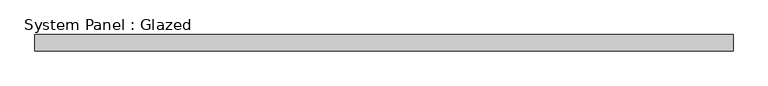
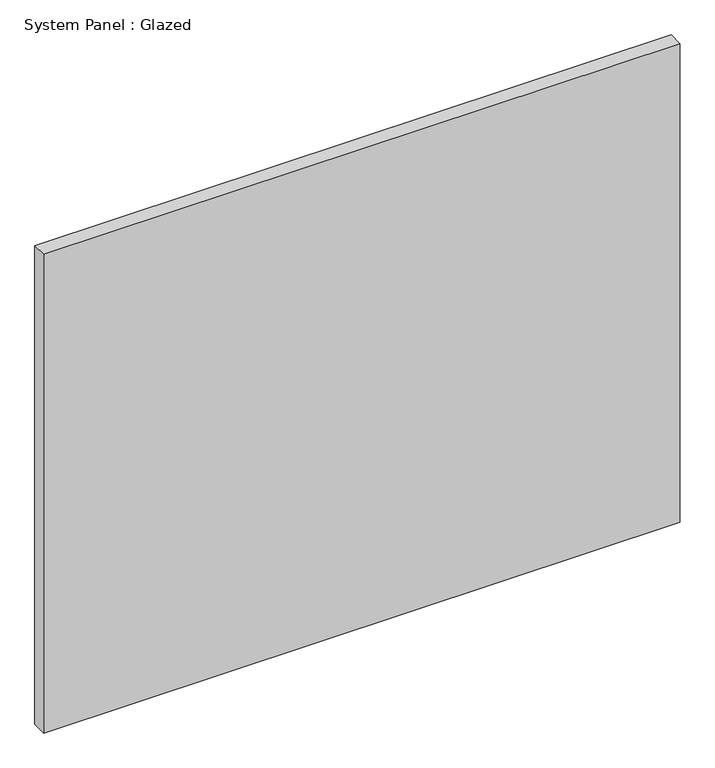
"""IFC4 building model written with IfcOpenShell, lengths in millimetres: plate geometry, System Panel : Glazed."""

from ifc_helpers import new_model, si_unit, origin, origin_with_axes, place, context, project, spatial, polyline, outline, extrude, source, transform, mapped, element, save


def system_panel_glazed_caa91b16(model_context):
    return source(origin(), model_context, "Body", "SweptSolid", [
        extrude(outline(polyline([(536.575, 19.05), (-536.575, 19.05), (-536.575, 44.45), (536.575, 44.45), (536.575, 19.05)])), origin_with_axes(), (0.0, 0.0, 1.0), 853.0145651),
    ])


if __name__ == "__main__":
    model = new_model("IFC4")
    model_context = context("Model", 3, world=origin())
    ifc_project = project(units=[si_unit("LENGTHUNIT", "METRE", prefix="MILLI")], contexts=[model_context])
    site = spatial("IfcSite", under=ifc_project)
    building = spatial("IfcBuilding", under=site)
    placement = place(None, origin())
    system_panel_glazed_shape = system_panel_glazed_caa91b16(model_context)
    element("IfcPlate", 1, ObjectType="System Panel : Glazed", at=placement, inside=building, context=model_context, shape_type="MappedRepresentation", body=[
        mapped(system_panel_glazed_shape, transform((0.0, 0.0, 0.0), x_axis=(1.0, 0.0, 0.0), y_axis=(0.0, 1.0, 0.0), z_axis=(0.0, 0.0, 1.0))),
    ])
    save(model, "model.ifc")

# Revit data of these elements
# Type "System Panel : Glazed"
#   Construction Type Id = "GSP4R"
#   Analytic Construction = "1/8 in Pilkington single glazing"
#   Visual Light Transmittance = 0.9
#   Solar Heat Gain Coefficient = 0.86
#   Heat Transfer Coefficient (U) = 1.18115 BTU/(h·ft²·°F)
#   Define Thermal Properties by = 1
# Element 1 (IfcPlate, "System Panel : Glazed")
#   Materials on its faces: "Glass"
# Materials
#   "Glass": class "Glass", colour RGB 0 128 192, transparency 0.75, Description = "Soda Lime Glass", Cost = 0
